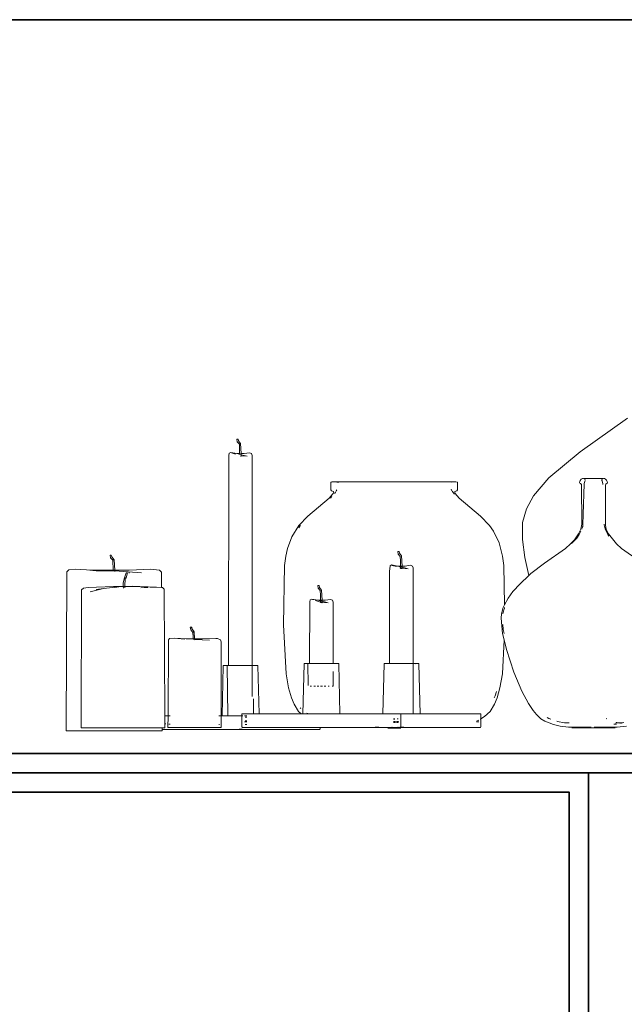
# Model space of a CAD drawing. Units: millimetres. Extents: x 446512 to 447461, y 70395 to 70610.
# Tile 7 of 39: x 446714 to 446730, y 70447 to 70473. Entities that reach past the tile are written whole.
import ezdxf

# ---------------------------------------------------------------- set-up
doc = ezdxf.new("R2010")
doc.units = ezdxf.units.MM
doc.layers.add('A-FURN', color=7, linetype='Continuous', lineweight=35)
doc.layers.add('A-FURN-DECO', color=8, linetype='Continuous', lineweight=13)

msp = doc.modelspace()

# ---------------------------------------------------------------- linework, layer by layer
at = {"layer": 'A-FURN'}
for p, q in [((446686.5728, 70453.3815), (446746.5728, 70453.3815)), ((446729.0084, 70453.3815), (446729.0084, 70433.3815))]:
    msp.add_line(p, q, dxfattribs=at)
for points in [[(446699.4288, 70473.3815), (446746.5728, 70473.3815), (446746.5728, 70453.3815), (446699.4288, 70453.3815)], [(446699.9288, 70472.8815), (446746.0728, 70472.8815), (446746.0728, 70453.8815), (446699.9288, 70453.8815)], [(446686.5728, 70453.3815), (446729.0084, 70453.3815), (446729.0084, 70433.3815), (446686.5728, 70433.3815)], [(446687.0728, 70452.8815), (446728.5084, 70452.8815), (446728.5084, 70433.8815), (446687.0728, 70433.8815)]]:
    msp.add_lwpolyline(points, close=True, dxfattribs=at)
at = {"layer": 'A-FURN-DECO'}
for p, q in [((446728.7945, 70461.6966), (446730.0171, 70462.5633)), ((446719.9441, 70462.0239), (446719.9104, 70462.0221)), ((446719.9188, 70461.9558), (446719.9104, 70462.0221)), ((446719.9756, 70461.8931), (446719.9188, 70461.9558)), ((446719.9519, 70461.9783), (446719.9441, 70462.0239)), ((446720.0049, 70461.9074), (446719.9519, 70461.9783)), ((446719.978, 70461.7795), (446719.9756, 70461.8931)), ((446719.9814, 70461.6492), (446719.978, 70461.7795)), ((446720.0049, 70461.9074), (446720.0223, 70461.6492)), ((446728.7945, 70461.6966), (446727.9781, 70461.0217)), ((446719.6988, 70456.1631), (446719.7022, 70461.6032)), ((446719.7022, 70461.6032), (446719.715, 70461.6578)), ((446719.7565, 70461.6773), (446719.715, 70461.6578)), ((446719.9071, 70461.6494), (446719.7565, 70461.6773)), ((446719.877, 70461.6334), (446719.7704, 70461.6668)), ((446719.7704, 70461.6668), (446719.9071, 70461.6494)), ((446719.9071, 70461.6494), (446719.9814, 70461.6492)), ((446719.982, 70461.63), (446719.9071, 70461.6494)), ((446719.982, 70461.63), (446719.9814, 70461.6492)), ((446720.0243, 70461.619), (446719.982, 70461.63)), ((446719.9821, 70461.6228), (446719.982, 70461.63)), ((446720.01, 70461.5841), (446720.0037, 70461.5844)), ((446720.008, 70461.6492), (446720.0199, 70461.6492)), ((446720.0098, 70461.5932), (446720.0261, 70461.5919)), ((446720.01, 70461.5841), (446720.0267, 70461.5837)), ((446720.0223, 70461.6492), (446720.1003, 70461.6491)), ((446720.0223, 70461.6492), (446720.0243, 70461.619)), ((446720.1784, 70461.5791), (446720.0243, 70461.619)), ((446720.0243, 70461.619), (446720.0256, 70461.5995)), ((446720.0261, 70461.5919), (446720.0267, 70461.5837)), ((446720.0261, 70461.5919), (446720.1784, 70461.5791)), ((446720.1003, 70461.6491), (446720.2369, 70461.6697)), ((446720.2369, 70461.6697), (446720.2923, 70461.6485)), ((446720.2923, 70461.6485), (446720.3052, 70461.5993)), ((446720.3089, 70456.1632), (446720.3052, 70461.5993)), ((446727.5827, 70460.5532), (446727.9781, 70461.0217)), ((446728.7887, 70460.9536), (446728.7747, 70460.9046)), ((446728.8207, 70460.9887), (446728.7887, 70460.9536)), ((446728.8499, 70461.0013), (446728.8207, 70460.9887)), ((446728.8772, 70461.0013), (446728.8499, 70461.0013)), ((446728.8976, 70460.9992), (446728.8772, 70461.0013)), ((446728.8961, 70460.8775), (446728.9208, 70460.9522)), ((446728.8976, 70460.9992), (446728.8991, 70461.0013)), ((446728.8976, 70460.9992), (446728.9159, 70460.9903)), ((446728.8991, 70461.0013), (446729.3721, 70461.0013)), ((446728.9202, 70460.9702), (446728.9159, 70460.9903)), ((446729.3502, 70460.9737), (446729.3477, 70460.9471)), ((446729.3492, 70460.9776), (446729.3509, 70460.9807)), ((446729.3502, 70460.9737), (446729.3492, 70460.9776)), ((446729.3578, 70460.9443), (446729.3502, 70460.9737)), ((446729.3525, 70460.9903), (446729.3508, 70460.9838)), ((446729.3524, 70460.9836), (446729.3569, 70460.992)), ((446729.3736, 70460.9992), (446729.3569, 70460.992)), ((446729.3749, 70460.8785), (446729.3592, 70460.9391)), ((446729.3721, 70461.0013), (446729.3736, 70460.9992)), ((446729.394, 70461.0013), (446729.3736, 70460.9992)), ((446729.4213, 70461.0013), (446729.394, 70461.0013)), ((446729.4459, 70460.9887), (446729.4213, 70461.0013)), ((446729.4459, 70460.9887), (446729.4757, 70460.9645)), ((446729.4925, 70460.9301), (446729.4757, 70460.9645)), ((446729.4925, 70460.9301), (446729.4961, 70460.8996)), ((446722.3491, 70460.9132), (446722.3421, 70460.8983)), ((446722.3453, 70460.7068), (446722.3421, 70460.8983)), ((446722.3453, 70460.7068), (446722.3571, 70460.686)), ((446722.3662, 70460.921), (446722.3491, 70460.9132)), ((446722.3571, 70460.686), (446722.4097, 70460.6657)), ((446722.4195, 70460.921), (446722.3662, 70460.921)), ((446722.3662, 70460.921), (446722.5008, 70460.9114)), ((446722.4311, 70460.922), (446722.4195, 70460.921)), ((446722.4311, 70460.922), (446722.6043, 70460.922)), ((446722.483, 70460.6864), (446722.4986, 70460.7139)), ((446722.5008, 70460.9114), (446722.5021, 70460.9106)), ((446722.5021, 70460.9106), (446722.5091, 70460.9063)), ((446722.5021, 70460.9106), (446722.5457, 70460.9072)), ((446722.5457, 70460.9072), (446722.5479, 70460.9073)), ((446722.8346, 70460.921), (446722.6043, 70460.922)), ((446722.8346, 70460.921), (446723.1792, 70460.921)), ((446723.1792, 70460.921), (446723.5625, 70460.922)), ((446723.5625, 70460.922), (446723.5688, 70460.922)), ((446723.5688, 70460.922), (446723.5748, 70460.922)), ((446723.5748, 70460.922), (446723.9747, 70460.921)), ((446724.4053, 70460.921), (446723.9747, 70460.921)), ((446724.7723, 70460.922), (446724.4053, 70460.921)), ((446724.7898, 70460.922), (446724.7723, 70460.922)), ((446724.7898, 70460.922), (446725.1125, 70460.922)), ((446725.3764, 70460.921), (446725.1125, 70460.922)), ((446725.3764, 70460.921), (446725.5426, 70460.921)), ((446725.452, 70460.9065), (446725.5746, 70460.922)), ((446725.4646, 70460.6981), (446725.4523, 70460.7241)), ((446725.4748, 70460.685), (446725.4646, 70460.6981)), ((446725.5446, 70460.5959), (446725.4822, 70460.6756)), ((446725.5426, 70460.921), (446725.5746, 70460.922)), ((446725.6029, 70460.684), (446725.5502, 70460.6636)), ((446725.5746, 70460.922), (446725.6171, 70460.9078)), ((446725.6169, 70460.7068), (446725.6029, 70460.684)), ((446725.6171, 70460.9078), (446725.6169, 70460.7068)), ((446728.7747, 70460.9046), (446728.7818, 70460.8831)), ((446728.7984, 70460.8735), (446728.7818, 70460.8831)), ((446728.7846, 70460.8865), (446728.7984, 70460.8735)), ((446728.7984, 70460.8735), (446728.8165, 70460.8563)), ((446728.8165, 70460.8563), (446728.8236, 70460.8453)), ((446728.8165, 70460.8563), (446728.8281, 70460.8453)), ((446728.8236, 70460.8453), (446728.8306, 70459.8199)), ((446728.8683, 70460.0694), (446728.8949, 70460.8628)), ((446728.8683, 70460.0694), (446728.898, 70460.862)), ((446729.3752, 70460.8691), (446729.3749, 70460.8785)), ((446729.3761, 70460.8439), (446729.3759, 70460.8497)), ((446729.4475, 70460.8431), (446729.444, 70459.7861)), ((446729.4475, 70460.8431), (446729.4529, 70460.8582)), ((446729.4529, 70460.8582), (446729.4894, 70460.8831)), ((446729.4894, 70460.8831), (446729.4961, 70460.8996)), ((446722.2982, 70460.4984), (446721.7473, 70460.0316)), ((446722.396, 70460.6047), (446722.2982, 70460.4984)), ((446722.3339, 70460.4984), (446722.3632, 70460.5266)), ((446722.3708, 70460.5354), (446722.3632, 70460.5266)), ((446722.416, 70460.6431), (446722.396, 70460.6047)), ((446722.4097, 70460.6657), (446722.416, 70460.6431)), ((446722.4502, 70460.6286), (446722.4382, 70460.6146)), ((446722.4502, 70460.6286), (446722.473, 70460.6689)), ((446725.5502, 70460.6636), (446725.5453, 70460.6516)), ((446725.5453, 70460.6516), (446725.5562, 70460.6199)), ((446725.5562, 70460.6199), (446725.664, 70460.4984)), ((446725.664, 70460.4984), (446726.2149, 70460.0316)), ((446727.4014, 70460.2208), (446727.5827, 70460.5532)), ((446727.4014, 70460.2208), (446727.3011, 70459.8693)), ((446721.7473, 70460.0316), (446721.5179, 70459.7851)), ((446726.2149, 70460.0316), (446726.4443, 70459.7851)), ((446728.8683, 70460.0694), (446728.8587, 70459.813)), ((446721.5179, 70459.7851), (446721.3347, 70459.4924)), ((446721.5131, 70459.7239), (446721.5432, 70459.7682)), ((446721.5432, 70459.7682), (446721.5573, 70459.7851)), ((446726.4443, 70459.7851), (446726.5455, 70459.6402)), ((446727.3011, 70459.8693), (446727.2951, 70459.4275)), ((446728.7483, 70459.5707), (446728.8051, 70459.6966)), ((446728.8306, 70459.8199), (446728.8051, 70459.6966)), ((446728.8368, 70459.6996), (446728.8326, 70459.6907)), ((446728.8575, 70459.7807), (446728.8409, 70459.715)), ((446728.8564, 70459.752), (446728.8575, 70459.7807)), ((446728.8588, 70459.786), (446728.8575, 70459.7807)), ((446728.8587, 70459.813), (446728.8588, 70459.786)), ((446729.4108, 70459.801), (446729.4101, 70459.8199)), ((446729.4338, 70459.7009), (446729.4108, 70459.801)), ((446729.5022, 70459.5548), (446729.4338, 70459.7009)), ((446729.444, 70459.7861), (446729.4661, 70459.6966)), ((446729.4661, 70459.6966), (446729.5229, 70459.5707)), ((446721.3347, 70459.4924), (446721.2205, 70459.1885)), ((446726.5455, 70459.6402), (446726.6922, 70459.3418)), ((446727.3592, 70458.9579), (446727.2951, 70459.4275)), ((446728.6407, 70459.4164), (446728.5404, 70459.3091)), ((446728.5656, 70459.3206), (446728.7087, 70459.464)), ((446728.6407, 70459.4164), (446728.7483, 70459.5707)), ((446728.769, 70459.5548), (446728.7087, 70459.464)), ((446728.8078, 70459.6377), (446728.769, 70459.5548)), ((446729.5334, 70459.513), (446729.5022, 70459.5548)), ((446729.5229, 70459.5707), (446729.7308, 70459.3091)), ((446721.2205, 70459.1885), (446721.1771, 70458.9933)), ((446726.6922, 70459.3418), (446726.7851, 70458.9933)), ((446728.4101, 70459.1958), (446727.8647, 70458.8154)), ((446728.5404, 70459.3091), (446728.4101, 70459.1958)), ((446729.8611, 70459.1958), (446729.7308, 70459.3091)), ((446730.4065, 70458.8154), (446729.8611, 70459.1958)), ((446716.6354, 70459.0201), (446716.6571, 70459.0212)), ((446716.6354, 70459.0201), (446716.6442, 70458.9513)), ((446716.6442, 70458.9513), (446716.7034, 70458.8861)), ((446716.6787, 70458.9748), (446716.6571, 70459.0212)), ((446716.6866, 70458.9642), (446716.6787, 70458.9748)), ((446716.7339, 70458.901), (446716.6866, 70458.9642)), ((446716.7224, 70458.8952), (446716.6866, 70458.9642)), ((446716.7034, 70458.8861), (446716.7224, 70458.8952)), ((446716.7224, 70458.8952), (446716.7339, 70458.901)), ((446716.752, 70458.632), (446716.7339, 70458.901)), ((446721.1771, 70458.9933), (446721.1469, 70458.754)), ((446724.1064, 70459.1159), (446724.0725, 70459.1141)), ((446724.0809, 70459.0472), (446724.0725, 70459.1141)), ((446724.1382, 70458.984), (446724.0809, 70459.0472)), ((446724.1143, 70459.0699), (446724.1064, 70459.1159)), ((446724.1678, 70458.9984), (446724.1143, 70459.0699)), ((446724.1406, 70458.8694), (446724.1382, 70458.984)), ((446724.1678, 70458.9984), (446724.1853, 70458.7377)), ((446726.7851, 70458.9933), (446726.8153, 70458.754)), ((446727.4673, 70458.4954), (446727.3592, 70458.9579)), ((446715.5105, 70458.5841), (446715.5626, 70458.641)), ((446715.5626, 70458.641), (446715.7315, 70458.6612)), ((446715.7315, 70458.6612), (446716.0257, 70458.6369)), ((446716.0257, 70458.6369), (446716.3433, 70458.6322)), ((446716.0257, 70458.6369), (446716.2746, 70458.615)), ((446716.3433, 70458.6322), (446716.7096, 70458.632)), ((446716.7034, 70458.8861), (446716.7096, 70458.632)), ((446716.7096, 70458.632), (446716.71, 70458.6145)), ((446716.7187, 70458.632), (446716.752, 70458.632)), ((446716.752, 70458.632), (446717.1286, 70458.6319)), ((446716.7533, 70458.6131), (446716.752, 70458.632)), ((446717.6839, 70458.6534), (446717.1286, 70458.6319)), ((446717.6839, 70458.6534), (446717.9093, 70458.6313)), ((446721.1469, 70458.754), (446721.119, 70457.2186)), ((446723.8582, 70458.5941), (446723.8754, 70458.7468)), ((446723.9173, 70458.7664), (446723.8754, 70458.7468)), ((446723.9173, 70458.7664), (446724.0691, 70458.7374)), ((446723.9313, 70458.7559), (446724.0691, 70458.7374)), ((446724.0388, 70458.7222), (446723.9313, 70458.7559)), ((446724.1441, 70458.7376), (446724.0691, 70458.7374)), ((446724.1446, 70458.7181), (446724.0691, 70458.7374)), ((446724.1454, 70458.6888), (446724.1244, 70458.6954)), ((446724.1441, 70458.7376), (446724.1406, 70458.8694)), ((446724.1853, 70458.7377), (446724.1441, 70458.7376)), ((446724.1446, 70458.7181), (446724.1441, 70458.7376)), ((446724.1448, 70458.7115), (446724.1446, 70458.7181)), ((446724.1873, 70458.7072), (446724.1446, 70458.7181)), ((446724.1454, 70458.6888), (446724.145, 70458.7021)), ((446724.1665, 70458.6822), (446724.1454, 70458.6888)), ((446724.1458, 70458.6738), (446724.1454, 70458.6888)), ((446724.1729, 70458.6724), (446724.1458, 70458.6738)), ((446724.1891, 70458.6803), (446724.1665, 70458.6822)), ((446724.1729, 70458.6724), (446724.1897, 70458.672)), ((446724.2639, 70458.7379), (446724.1853, 70458.7377)), ((446724.1853, 70458.7377), (446724.1873, 70458.7072)), ((446724.1873, 70458.7072), (446724.1886, 70458.6881)), ((446724.3427, 70458.6674), (446724.1873, 70458.7072)), ((446724.1891, 70458.6803), (446724.1897, 70458.672)), ((446724.3427, 70458.6674), (446724.1891, 70458.6803)), ((446724.4017, 70458.7588), (446724.2639, 70458.7379)), ((446724.4576, 70458.7374), (446724.4017, 70458.7588)), ((446724.4705, 70458.6877), (446724.4576, 70458.7374)), ((446724.4724, 70456.2151), (446724.4705, 70458.6877)), ((446726.8153, 70458.754), (446726.8338, 70457.7327)), ((446727.5189, 70458.543), (446727.8647, 70458.8154)), ((446715.4932, 70454.4707), (446715.5105, 70458.5841)), ((446716.2746, 70458.615), (446716.2883, 70458.6148)), ((446716.2883, 70458.6148), (446716.71, 70458.6145)), ((446716.71, 70458.6145), (446716.7359, 70458.6145)), ((446716.7359, 70458.6145), (446716.7533, 70458.6131)), ((446716.7533, 70458.6131), (446717.4462, 70458.559)), ((446716.7541, 70458.6003), (446716.7533, 70458.6131)), ((446716.9685, 70458.3005), (446717.004, 70458.4341)), ((446717.004, 70458.4341), (446717.0495, 70458.5607)), ((446717.0229, 70458.425), (446717.0178, 70458.2115)), ((446717.0245, 70458.4398), (446717.0229, 70458.425)), ((446717.0229, 70458.425), (446717.042, 70458.425)), ((446717.042, 70458.425), (446717.0475, 70458.434)), ((446717.0475, 70458.434), (446717.0856, 70458.56)), ((446717.0495, 70458.5607), (446717.0856, 70458.56)), ((446717.1161, 70458.5661), (446717.1347, 70458.5657)), ((446717.9614, 70458.58), (446717.9093, 70458.6313)), ((446717.963, 70458.1808), (446717.9614, 70458.58)), ((446723.8582, 70456.2151), (446723.8582, 70458.5941)), ((446727.2355, 70458.2815), (446727.4673, 70458.4954)), ((446727.4673, 70458.4954), (446727.5189, 70458.543)), ((446715.8817, 70454.5456), (446715.8968, 70458.1227)), ((446715.9421, 70458.1689), (446715.8968, 70458.1227)), ((446716.0693, 70458.1802), (446715.9421, 70458.1689)), ((446716.7205, 70458.2113), (446716.0693, 70458.1802)), ((446716.1194, 70458.0708), (446716.4619, 70458.1529)), ((446716.2717, 70458.1312), (446716.4619, 70458.1529)), ((446716.8597, 70458.2036), (446716.4619, 70458.1529)), ((446716.7205, 70458.2113), (446716.9736, 70458.2114)), ((446716.759, 70458.1855), (446716.8597, 70458.2036)), ((446716.8597, 70458.2036), (446716.9738, 70458.207)), ((446716.9736, 70458.2114), (446716.9685, 70458.3005)), ((446716.9736, 70458.2114), (446716.9777, 70458.2114)), ((446716.9738, 70458.207), (446716.9736, 70458.2114)), ((446716.9738, 70458.207), (446717.0177, 70458.2083)), ((446716.9761, 70458.1671), (446716.9738, 70458.207)), ((446717.0004, 70458.2115), (446717.0178, 70458.2115)), ((446717.0177, 70458.2083), (446717.0167, 70458.1721)), ((446717.0177, 70458.2083), (446717.1242, 70458.2115)), ((446717.0178, 70458.2115), (446717.0177, 70458.2083)), ((446717.0178, 70458.2115), (446717.1242, 70458.2115)), ((446717.1242, 70458.2115), (446717.2075, 70458.214)), ((446717.1242, 70458.2115), (446717.2775, 70458.2116)), ((446717.2075, 70458.214), (446717.2775, 70458.2116)), ((446717.2775, 70458.2116), (446717.7488, 70458.1951)), ((446717.2775, 70458.2116), (446717.4044, 70458.2116)), ((446717.4044, 70458.2116), (446717.8303, 70458.1954)), ((446717.4299, 70458.1719), (446717.6043, 70458.1821)), ((446717.6751, 70458.1863), (446717.8303, 70458.1954)), ((446717.8303, 70458.1954), (446717.7488, 70458.1951)), ((446717.8303, 70458.1954), (446717.963, 70458.1808)), ((446717.963, 70458.1808), (446717.9858, 70458.1808)), ((446717.9858, 70458.1808), (446718.0312, 70458.1354)), ((446718.0312, 70458.1354), (446718.045, 70454.8578)), ((446722.0386, 70458.2326), (446722.0047, 70458.2307)), ((446722.0131, 70458.164), (446722.0047, 70458.2307)), ((446722.0702, 70458.1009), (446722.0131, 70458.164)), ((446722.0464, 70458.1866), (446722.0386, 70458.2326)), ((446722.0998, 70458.1153), (446722.0464, 70458.1866)), ((446727.0519, 70458.0782), (446727.2355, 70458.2815)), ((446721.808, 70457.8642), (446721.8498, 70457.8837)), ((446721.8498, 70457.8837), (446722.0013, 70457.8556)), ((446721.8638, 70457.8732), (446722.0013, 70457.8556)), ((446722.0726, 70457.9866), (446722.0702, 70458.1009)), ((446722.0761, 70457.8555), (446722.0726, 70457.9866)), ((446722.0998, 70458.1153), (446722.1172, 70457.8555)), ((446722.1957, 70457.8554), (446722.3332, 70457.8761)), ((446722.389, 70457.8548), (446722.3332, 70457.8761)), ((446726.9252, 70457.9066), (446726.8338, 70457.7327)), ((446727.0519, 70458.0782), (446726.9252, 70457.9066)), ((446721.792, 70456.2151), (446721.7951, 70457.8092)), ((446721.7951, 70457.8092), (446721.808, 70457.8642)), ((446721.9427, 70457.8485), (446722.0774, 70457.8063)), ((446722.0013, 70457.8556), (446722.0761, 70457.8555)), ((446722.0013, 70457.8556), (446722.0766, 70457.8361)), ((446722.0761, 70457.8555), (446722.1172, 70457.8555)), ((446722.0766, 70457.8361), (446722.0761, 70457.8555)), ((446722.0766, 70457.8361), (446722.1192, 70457.8251)), ((446722.0774, 70457.8063), (446722.0766, 70457.8361)), ((446722.0774, 70457.8063), (446722.0985, 70457.7997)), ((446722.0778, 70457.7914), (446722.0774, 70457.8063)), ((446722.1049, 70457.79), (446722.0778, 70457.7914)), ((446722.1211, 70457.7978), (446722.0985, 70457.7997)), ((446722.1049, 70457.79), (446722.1216, 70457.7896)), ((446722.1172, 70457.8555), (446722.1957, 70457.8554)), ((446722.1172, 70457.8555), (446722.1192, 70457.8251)), ((446722.1192, 70457.8251), (446722.2743, 70457.7849)), ((446722.1192, 70457.8251), (446722.1211, 70457.7978)), ((446722.2743, 70457.7849), (446722.1211, 70457.7978)), ((446722.1211, 70457.7978), (446722.1216, 70457.7896)), ((446722.4019, 70457.8053), (446722.389, 70457.8548)), ((446722.4019, 70457.8053), (446722.405, 70456.2151)), ((446726.7531, 70457.4982), (446726.7992, 70457.6668)), ((446726.8338, 70457.7327), (446726.7992, 70457.6668)), ((446726.8355, 70457.6426), (446726.8171, 70457.6055)), ((446726.835, 70457.6668), (446726.837, 70457.6484)), ((446726.837, 70457.6484), (446726.8354, 70457.6449)), ((446726.8354, 70457.6449), (446726.8355, 70457.6426)), ((446726.7448, 70457.3867), (446726.7531, 70457.4982)), ((446726.7448, 70457.3867), (446726.7852, 70456.9946)), ((446726.7902, 70457.4982), (446726.8171, 70457.6055)), ((446718.7295, 70457.1576), (446718.7075, 70457.1558)), ((446718.7164, 70457.0871), (446718.7075, 70457.1558)), ((446718.7295, 70457.1576), (446718.7428, 70457.1581)), ((446718.7495, 70457.1187), (446718.7295, 70457.1576)), ((446718.7495, 70457.1187), (446718.7428, 70457.1581)), ((446718.7509, 70457.1106), (446718.7495, 70457.1187)), ((446718.7598, 70457.0987), (446718.7495, 70457.1187)), ((446718.7598, 70457.0987), (446718.7509, 70457.1106)), ((446721.119, 70457.2186), (446721.1834, 70455.9479)), ((446726.7872, 70457.222), (446726.8035, 70457.0922)), ((446718.1394, 70456.8302), (446718.1682, 70456.8616)), ((446718.2925, 70456.8668), (446718.1682, 70456.8616)), ((446718.5676, 70456.8447), (446718.2925, 70456.8668)), ((446718.5988, 70456.8568), (446718.2925, 70456.8668)), ((446718.2925, 70456.8668), (446718.7797, 70456.8412)), ((446718.7793, 70456.8567), (446718.5988, 70456.8568)), ((446718.7164, 70457.0871), (446718.7756, 70457.0219)), ((446718.7946, 70457.031), (446718.7598, 70457.0987)), ((446718.8061, 70457.0368), (446718.7598, 70457.0987)), ((446718.7946, 70457.031), (446718.7756, 70457.0219)), ((446718.7784, 70456.9061), (446718.7756, 70457.0219)), ((446718.778, 70456.9035), (446718.7784, 70456.9061)), ((446718.778, 70456.9035), (446718.7793, 70456.8567)), ((446718.7793, 70456.8567), (446718.7797, 70456.8412)), ((446718.8182, 70456.8567), (446718.7793, 70456.8567)), ((446718.8061, 70457.0368), (446718.7946, 70457.031)), ((446718.8182, 70456.8567), (446718.8061, 70457.0368)), ((446718.8193, 70456.8398), (446718.8182, 70456.8567)), ((446719.0321, 70456.8566), (446718.8182, 70456.8567)), ((446719.3696, 70456.8619), (446719.0321, 70456.8566)), ((446719.4116, 70456.8598), (446719.3696, 70456.8619)), ((446719.4915, 70456.828), (446719.4116, 70456.8598)), ((446726.8235, 70456.8308), (446726.7852, 70456.9946)), ((446726.8035, 70457.0922), (446726.8258, 70456.9946)), ((446718.1311, 70454.8578), (446718.1394, 70456.8302)), ((446718.7797, 70456.8412), (446718.8155, 70456.8401)), ((446718.8193, 70456.8398), (446718.8155, 70456.8401)), ((446719.2073, 70456.8164), (446718.8193, 70456.8398)), ((446718.8214, 70456.8095), (446718.8213, 70456.8112)), ((446719.5011, 70456.7748), (446719.4915, 70456.828)), ((446719.5011, 70456.7748), (446719.5011, 70454.8578)), ((446726.8235, 70456.8308), (446726.7788, 70455.9479)), ((446726.8836, 70456.5742), (446726.8235, 70456.8308)), ((446727.0748, 70455.9925), (446726.8836, 70456.5742)), ((446719.5279, 70454.8578), (446719.5578, 70456.1587)), ((446719.5578, 70456.1587), (446719.563, 70456.1631)), ((446719.5894, 70456.1631), (446719.563, 70456.1631)), ((446719.5973, 70456.1632), (446719.5894, 70456.1631)), ((446719.6042, 70456.1631), (446719.5973, 70456.1632)), ((446719.6064, 70456.1631), (446719.6042, 70456.1631)), ((446719.6089, 70456.1632), (446719.6064, 70456.1631)), ((446719.6245, 70456.1631), (446719.6089, 70456.1632)), ((446719.6245, 70456.1631), (446719.6397, 70456.1632)), ((446719.6397, 70456.1632), (446719.6479, 70456.1632)), ((446719.6479, 70456.1632), (446719.6517, 70456.1631)), ((446719.6517, 70456.1631), (446719.6576, 70456.1632)), ((446719.6576, 70456.1632), (446719.6768, 70454.8578)), ((446719.6576, 70456.1632), (446719.6674, 70456.1632)), ((446719.6761, 70456.1631), (446719.6674, 70456.1632)), ((446719.6783, 70456.1632), (446719.6761, 70456.1631)), ((446719.6988, 70456.1631), (446719.6783, 70456.1632)), ((446719.6988, 70456.1631), (446719.708, 70456.1632)), ((446719.6988, 70456.1587), (446719.6988, 70456.1631)), ((446719.708, 70456.1632), (446719.7106, 70456.1631)), ((446719.7106, 70456.1631), (446719.7228, 70456.1631)), ((446719.7228, 70456.1631), (446719.7272, 70456.1632)), ((446719.7272, 70456.1632), (446719.7304, 70456.1632)), ((446719.7304, 70456.1632), (446719.7469, 70456.1632)), ((446719.7574, 70456.1632), (446719.7469, 70456.1632)), ((446719.7574, 70456.1632), (446719.7735, 70456.1632)), ((446719.7766, 70456.1631), (446719.7735, 70456.1632)), ((446719.7794, 70456.1632), (446719.7766, 70456.1631)), ((446719.781, 70456.1631), (446719.7794, 70456.1632)), ((446719.7832, 70456.1632), (446719.781, 70456.1631)), ((446719.7881, 70456.1631), (446719.7832, 70456.1632)), ((446719.7881, 70456.1631), (446719.8002, 70456.1632)), ((446719.8196, 70456.1631), (446719.8002, 70456.1632)), ((446719.8196, 70456.1631), (446719.8593, 70456.1632)), ((446719.9019, 70456.1631), (446719.8593, 70456.1632)), ((446719.9019, 70456.1631), (446719.9241, 70456.1632)), ((446719.9241, 70456.1632), (446719.9883, 70456.1631)), ((446719.9883, 70456.1631), (446719.992, 70456.1632)), ((446719.992, 70456.1632), (446720.0264, 70456.1632)), ((446720.032, 70456.1631), (446720.0264, 70456.1632)), ((446720.032, 70456.1631), (446720.0943, 70456.1632)), ((446720.1182, 70456.1631), (446720.0943, 70456.1632)), ((446720.1182, 70456.1631), (446720.1588, 70456.1632)), ((446720.2002, 70456.1631), (446720.1588, 70456.1632)), ((446720.2002, 70456.1631), (446720.2176, 70456.1632)), ((446720.2176, 70456.1632), (446720.2386, 70456.1631)), ((446720.2386, 70456.1631), (446720.2682, 70456.1632)), ((446720.2682, 70456.1632), (446720.2754, 70456.1632)), ((446720.2941, 70456.1632), (446720.2754, 70456.1632)), ((446720.2941, 70456.1632), (446720.3038, 70456.1631)), ((446720.3038, 70456.1631), (446720.3089, 70456.1632)), ((446720.3091, 70455.3578), (446720.3089, 70456.1632)), ((446720.3115, 70456.1632), (446720.3089, 70456.1632)), ((446720.3207, 70456.1632), (446720.3115, 70456.1632)), ((446720.3222, 70456.1632), (446720.3207, 70456.1632)), ((446720.3235, 70456.1632), (446720.3222, 70456.1632)), ((446720.3235, 70456.1632), (446720.3249, 70456.1632)), ((446720.3296, 70456.1632), (446720.3249, 70456.1632)), ((446720.331, 70456.1632), (446720.3296, 70456.1632)), ((446720.3333, 70456.1632), (446720.331, 70456.1632)), ((446720.3356, 70456.1631), (446720.3333, 70456.1632)), ((446720.339, 70456.1631), (446720.3356, 70456.1631)), ((446720.3427, 70456.1632), (446720.339, 70456.1631)), ((446720.3444, 70456.1632), (446720.3427, 70456.1632)), ((446720.3444, 70456.1632), (446720.3478, 70456.1632)), ((446720.3456, 70456.1632), (446720.3444, 70456.1632)), ((446720.3478, 70456.1632), (446720.3456, 70456.1632)), ((446720.3478, 70456.1632), (446720.3503, 70456.1632)), ((446720.3538, 70456.1632), (446720.3503, 70456.1632)), ((446720.3575, 70456.1632), (446720.3538, 70456.1632)), ((446720.3575, 70456.1632), (446720.3575, 70456.1587)), ((446720.361, 70456.1632), (446720.3575, 70456.1632)), ((446720.3635, 70456.1631), (446720.361, 70456.1632)), ((446720.3809, 70456.1632), (446720.3635, 70456.1631)), ((446720.3872, 70456.1632), (446720.3809, 70456.1632)), ((446720.3906, 70456.1631), (446720.3872, 70456.1632)), ((446720.3926, 70456.1632), (446720.3906, 70456.1631)), ((446720.3926, 70456.1632), (446720.452, 70456.1631)), ((446720.4574, 70456.1587), (446720.452, 70456.1631)), ((446720.4861, 70454.9097), (446720.4574, 70456.1587)), ((446721.6183, 70454.9097), (446721.6482, 70456.2106)), ((446721.6482, 70456.2106), (446721.6536, 70456.2151)), ((446721.6536, 70456.2151), (446721.7072, 70456.2151)), ((446721.7072, 70456.2151), (446721.7119, 70456.2151)), ((446721.7119, 70456.2151), (446721.7149, 70456.2151)), ((446721.7149, 70456.2151), (446721.7175, 70456.2151)), ((446721.7175, 70456.2151), (446721.7188, 70456.2151)), ((446721.7188, 70456.2151), (446721.726, 70456.2151)), ((446721.726, 70456.2151), (446721.739, 70456.2151)), ((446721.739, 70456.2151), (446721.741, 70456.2152)), ((446721.741, 70456.2152), (446721.7438, 70456.2151)), ((446721.7438, 70456.2151), (446721.7481, 70456.2152)), ((446721.7481, 70456.2152), (446721.7565, 70455.6418)), ((446721.7481, 70456.2152), (446721.7585, 70456.2152)), ((446721.7585, 70456.2152), (446721.7699, 70456.2151)), ((446721.7699, 70456.2151), (446721.7806, 70456.2152)), ((446721.7806, 70456.2152), (446721.782, 70456.2152)), ((446721.7901, 70456.2151), (446721.782, 70456.2152)), ((446721.792, 70456.2151), (446721.7901, 70456.2151)), ((446721.792, 70456.2106), (446721.792, 70456.2151)), ((446721.792, 70456.2151), (446721.8162, 70456.2151)), ((446721.8162, 70456.2151), (446721.8176, 70456.2152)), ((446721.8176, 70456.2152), (446721.8639, 70456.2152)), ((446721.8713, 70456.2151), (446721.8639, 70456.2152)), ((446721.8713, 70456.2151), (446721.8906, 70456.2152)), ((446721.9923, 70456.2151), (446721.8906, 70456.2152)), ((446721.9923, 70456.2151), (446722.0144, 70456.2152)), ((446722.0787, 70456.2151), (446722.0144, 70456.2152)), ((446722.0787, 70456.2151), (446722.0824, 70456.2152)), ((446722.0824, 70456.2152), (446722.1168, 70456.2152)), ((446722.1223, 70456.2151), (446722.1168, 70456.2152)), ((446722.1223, 70456.2151), (446722.1847, 70456.2152)), ((446722.2086, 70456.2151), (446722.1847, 70456.2152)), ((446722.3079, 70456.2152), (446722.2086, 70456.2151)), ((446722.3079, 70456.2152), (446722.3289, 70456.2151)), ((446722.3289, 70456.2151), (446722.3344, 70456.2152)), ((446722.3344, 70456.2152), (446722.3807, 70456.2151)), ((446722.3807, 70456.2151), (446722.405, 70456.2151)), ((446722.405, 70456.2151), (446722.405, 70456.2106)), ((446722.4294, 70456.2151), (446722.405, 70456.2151)), ((446722.4294, 70456.2151), (446722.4321, 70456.2151)), ((446722.4321, 70456.2151), (446722.4341, 70456.2151)), ((446722.4341, 70456.2151), (446722.4442, 70456.2152)), ((446722.4479, 70456.2152), (446722.4442, 70456.2152)), ((446722.4479, 70456.2152), (446722.4478, 70456.2106)), ((446722.4783, 70456.2151), (446722.4479, 70456.2152)), ((446722.4783, 70456.2151), (446722.481, 70456.2151)), ((446722.487, 70456.2151), (446722.481, 70456.2151)), ((446722.4992, 70456.2151), (446722.487, 70456.2151)), ((446722.4992, 70456.2151), (446722.5426, 70456.2151)), ((446722.5477, 70456.2106), (446722.5426, 70456.2151)), ((446722.5776, 70454.9097), (446722.5477, 70456.2106)), ((446723.6892, 70454.9097), (446723.7191, 70456.2106)), ((446723.7191, 70456.2106), (446723.7245, 70456.2151)), ((446723.7245, 70456.2151), (446723.7786, 70456.2151)), ((446723.7834, 70456.2151), (446723.7786, 70456.2151)), ((446723.8032, 70456.2151), (446723.7834, 70456.2151)), ((446723.8099, 70456.2151), (446723.8032, 70456.2151)), ((446723.813, 70456.2151), (446723.8099, 70456.2151)), ((446723.8191, 70456.2152), (446723.813, 70456.2151)), ((446723.8191, 70456.2152), (446723.819, 70456.2106)), ((446723.8191, 70456.2152), (446723.8295, 70456.2152)), ((446723.8374, 70456.2151), (446723.8295, 70456.2152)), ((446723.8435, 70456.2152), (446723.8374, 70456.2151)), ((446723.8515, 70456.2152), (446723.8435, 70456.2152)), ((446723.8529, 70456.2152), (446723.8515, 70456.2152)), ((446723.8582, 70456.2151), (446723.8529, 70456.2152)), ((446723.8676, 70456.2152), (446723.8582, 70456.2151)), ((446723.8582, 70456.2106), (446723.8582, 70456.2151)), ((446723.8719, 70456.2151), (446723.8676, 70456.2152)), ((446723.8719, 70456.2151), (446723.878, 70456.2151)), ((446723.878, 70456.2151), (446723.884, 70456.2151)), ((446723.884, 70456.2151), (446723.8885, 70456.2152)), ((446723.8885, 70456.2152), (446723.9058, 70456.2151)), ((446723.9058, 70456.2151), (446723.9104, 70456.2152)), ((446723.9104, 70456.2152), (446723.9485, 70456.2151)), ((446723.9485, 70456.2151), (446723.9589, 70456.2152)), ((446723.9589, 70456.2152), (446723.9615, 70456.2152)), ((446723.9809, 70456.2151), (446723.9615, 70456.2152)), ((446723.9809, 70456.2151), (446723.9902, 70456.2152)), ((446724.0099, 70456.2151), (446723.9902, 70456.2152)), ((446724.0099, 70456.2151), (446724.0524, 70456.2152)), ((446724.0632, 70456.2151), (446724.0524, 70456.2152)), ((446724.0632, 70456.2151), (446724.1191, 70456.2152)), ((446724.1496, 70456.2151), (446724.1191, 70456.2152)), ((446724.1496, 70456.2151), (446724.1877, 70456.2152)), ((446724.2367, 70456.2151), (446724.1877, 70456.2152)), ((446724.2367, 70456.2151), (446724.2556, 70456.2152)), ((446724.2556, 70456.2152), (446724.3201, 70456.2152)), ((446724.3218, 70456.2151), (446724.3201, 70456.2152)), ((446724.3218, 70456.2151), (446724.3476, 70456.2152)), ((446724.3476, 70456.2152), (446724.3698, 70456.2151)), ((446724.3789, 70456.2152), (446724.3698, 70456.2151)), ((446724.3833, 70456.2151), (446724.3789, 70456.2152)), ((446724.3833, 70456.2151), (446724.3999, 70456.2151)), ((446724.3999, 70456.2151), (446724.4295, 70456.2152)), ((446724.464, 70456.2151), (446724.4295, 70456.2152)), ((446724.4659, 70456.2151), (446724.464, 70456.2151)), ((446724.4697, 70456.2151), (446724.4659, 70456.2151)), ((446724.4724, 70456.2151), (446724.4697, 70456.2151)), ((446724.4734, 70454.9097), (446724.4724, 70456.2151)), ((446724.4752, 70456.2151), (446724.4724, 70456.2151)), ((446724.4778, 70456.2151), (446724.4752, 70456.2151)), ((446724.4793, 70456.2151), (446724.4778, 70456.2151)), ((446724.4831, 70456.2151), (446724.4793, 70456.2151)), ((446724.4849, 70456.2152), (446724.4831, 70456.2151)), ((446724.4873, 70456.2151), (446724.4849, 70456.2152)), ((446724.489, 70456.2151), (446724.4873, 70456.2151)), ((446724.4969, 70456.2151), (446724.489, 70456.2151)), ((446724.4993, 70456.2152), (446724.4969, 70456.2151)), ((446724.4993, 70456.2152), (446724.5018, 70456.2151)), ((446724.5018, 70456.2151), (446724.5152, 70456.2152)), ((446724.5189, 70456.2152), (446724.5152, 70456.2152)), ((446724.5189, 70456.2152), (446724.5188, 70456.2106)), ((446724.5279, 70456.2151), (446724.5189, 70456.2152)), ((446724.5303, 70456.2151), (446724.5279, 70456.2151)), ((446724.5342, 70456.2151), (446724.5303, 70456.2151)), ((446724.5365, 70456.2152), (446724.5342, 70456.2151)), ((446724.5493, 70456.2151), (446724.5365, 70456.2152)), ((446724.5613, 70456.2151), (446724.5493, 70456.2151)), ((446724.5668, 70456.2151), (446724.5613, 70456.2151)), ((446724.5668, 70456.2151), (446724.6133, 70456.2151)), ((446724.6187, 70456.2106), (446724.6133, 70456.2151)), ((446724.6486, 70454.9097), (446724.6187, 70456.2106)), ((446721.1834, 70455.9479), (446721.2475, 70455.5851)), ((446722.4054, 70456.007), (446722.4061, 70455.6258)), ((446726.7788, 70455.9479), (446726.7147, 70455.5851)), ((446727.0748, 70455.9925), (446727.2856, 70455.4981)), ((446721.2475, 70455.5851), (446721.3203, 70455.3274)), ((446721.8034, 70455.6258), (446721.8399, 70455.6258)), ((446721.9443, 70455.6258), (446721.9022, 70455.6258)), ((446722.0326, 70455.6258), (446721.9879, 70455.6258)), ((446722.0779, 70455.6258), (446722.1234, 70455.6258)), ((446722.2133, 70455.6258), (446722.1687, 70455.6258)), ((446722.2987, 70455.6258), (446722.2743, 70455.6258)), ((446722.4061, 70455.6258), (446722.3763, 70455.6258)), ((446726.7147, 70455.5851), (446726.6419, 70455.3274)), ((446721.3203, 70455.3274), (446721.3893, 70455.1589)), ((446726.5668, 70455.3274), (446726.592, 70455.3759)), ((446726.6419, 70455.3274), (446726.5729, 70455.1589)), ((446726.592, 70455.3759), (446726.6307, 70455.4902)), ((446727.4568, 70455.1775), (446727.2856, 70455.4981)), ((446720.3449, 70455.3023), (446720.3391, 70454.9097)), ((446721.3893, 70455.1589), (446721.5027, 70454.9746)), ((446721.5697, 70455.0499), (446721.5495, 70455.0689)), ((446726.5729, 70455.1589), (446726.4595, 70454.9746)), ((446727.4568, 70455.1775), (446727.5727, 70455.0013)), ((446718.045, 70454.8578), (446718.0459, 70454.6495)), ((446718.045, 70454.8578), (446718.1311, 70454.8578)), ((446718.1299, 70454.561), (446718.1311, 70454.8578)), ((446718.1311, 70454.8578), (446718.1852, 70454.8578)), ((446719.4457, 70454.8578), (446719.5011, 70454.8578)), ((446719.5011, 70454.8578), (446719.5011, 70454.561)), ((446719.5011, 70454.8578), (446719.5279, 70454.8578)), ((446719.5279, 70454.8578), (446719.6768, 70454.8578)), ((446720.0427, 70454.8578), (446719.6768, 70454.8578)), ((446720.0423, 70454.5773), (446720.0427, 70454.8578)), ((446720.0427, 70454.8578), (446720.0428, 70454.9097)), ((446720.0427, 70454.8578), (446720.0661, 70454.8578)), ((446720.0428, 70454.9097), (446720.0608, 70454.9097)), ((446720.0636, 70454.9096), (446720.0608, 70454.9097)), ((446720.0636, 70454.9096), (446720.0662, 70454.9097)), ((446720.0662, 70454.9097), (446720.0666, 70454.9064)), ((446720.0662, 70454.9097), (446720.1073, 70454.9097)), ((446720.1675, 70454.8578), (446720.1072, 70454.8578)), ((446720.1073, 70454.9097), (446720.1187, 70454.9096)), ((446720.1187, 70454.9096), (446720.1275, 70454.9096)), ((446720.1272, 70454.8261), (446720.1675, 70454.8261)), ((446720.1275, 70454.9096), (446720.1553, 70454.9097)), ((446720.3391, 70454.9097), (446720.1553, 70454.9097)), ((446720.4861, 70454.9097), (446720.3391, 70454.9097)), ((446721.571, 70454.9097), (446720.4861, 70454.9097)), ((446721.5027, 70454.9746), (446721.571, 70454.9097)), ((446721.571, 70454.9097), (446721.6183, 70454.9097)), ((446722.5776, 70454.9097), (446721.6183, 70454.9097)), ((446721.7443, 70454.9174), (446721.7225, 70454.929)), ((446723.6892, 70454.9097), (446722.5776, 70454.9097)), ((446723.9662, 70454.9097), (446723.6892, 70454.9097)), ((446723.9702, 70454.9118), (446723.9662, 70454.9097)), ((446723.9702, 70454.9118), (446723.9663, 70454.9112)), ((446723.9752, 70454.9097), (446723.9702, 70454.9118)), ((446723.9752, 70454.9097), (446723.9914, 70454.9097)), ((446723.9914, 70454.9097), (446724.0051, 70454.9118)), ((446724.0051, 70454.9118), (446724.0099, 70454.9097)), ((446724.0051, 70454.9118), (446724.0099, 70454.9118)), ((446724.0099, 70454.9097), (446724.0406, 70454.9097)), ((446724.0406, 70454.9097), (446724.0684, 70454.9096)), ((446724.0772, 70454.9096), (446724.0684, 70454.9096)), ((446724.0772, 70454.9096), (446724.0862, 70454.9097)), ((446724.1531, 70454.9097), (446724.0862, 70454.9097)), ((446724.1536, 70454.5773), (446724.1531, 70454.9097)), ((446724.1531, 70454.9097), (446724.4734, 70454.9097)), ((446724.4734, 70454.9097), (446724.6486, 70454.9097)), ((446724.6486, 70454.9097), (446726.1116, 70454.9097)), ((446726.1116, 70454.9097), (446726.1394, 70454.9096)), ((446726.1482, 70454.9096), (446726.1394, 70454.9096)), ((446726.1595, 70454.9097), (446726.1482, 70454.9096)), ((446726.1595, 70454.9097), (446726.224, 70454.9097)), ((446726.2242, 70454.782), (446726.224, 70454.9097)), ((446726.3186, 70454.8408), (446726.2242, 70454.782)), ((446726.4595, 70454.9746), (446726.3186, 70454.8408)), ((446727.6589, 70454.8939), (446727.5727, 70455.0013)), ((446727.7744, 70454.7867), (446727.6589, 70454.8939)), ((446727.9786, 70454.795), (446727.9403, 70454.8208)), ((446718.0459, 70454.6495), (446718.0769, 70454.6493)), ((446718.0459, 70454.6495), (446718.0463, 70454.5456)), ((446719.5011, 70454.561), (446718.1299, 70454.561)), ((446718.1558, 70454.6488), (446718.1844, 70454.6486)), ((446719.4466, 70454.64), (446719.4588, 70454.6399)), ((446720.058, 70454.5585), (446720.0423, 70454.5773)), ((446720.1819, 70454.5585), (446720.058, 70454.5585)), ((446720.107, 70454.7016), (446720.1566, 70454.7016)), ((446720.1672, 70454.6399), (446720.1268, 70454.6399)), ((446720.1657, 70454.7229), (446720.1273, 70454.7229)), ((446720.1278, 70454.7293), (446720.1437, 70454.7289)), ((446720.1278, 70454.7277), (446720.1437, 70454.7289)), ((446720.1657, 70454.7229), (446720.1278, 70454.7242)), ((446720.1437, 70454.7289), (446720.1495, 70454.7293)), ((446720.1495, 70454.7293), (446720.1673, 70454.7282)), ((446720.1566, 70454.7016), (446720.1673, 70454.7015)), ((446720.1673, 70454.7229), (446720.1657, 70454.7229)), ((446720.1819, 70454.5585), (446720.2586, 70454.5588)), ((446720.2602, 70454.5585), (446720.2586, 70454.5588)), ((446720.2602, 70454.5585), (446722.0632, 70454.5585)), ((446722.0632, 70454.5254), (446722.0632, 70454.5585)), ((446722.0632, 70454.5585), (446723.4982, 70454.5585)), ((446723.4833, 70454.5601), (446723.4982, 70454.5585)), ((446723.6009, 70454.5617), (446723.484, 70454.5614)), ((446723.4858, 70454.5646), (446723.5832, 70454.5643)), ((446723.5284, 70454.5587), (446723.4982, 70454.5585)), ((446723.6009, 70454.5617), (446723.5284, 70454.5587)), ((446723.5984, 70454.5585), (446723.5284, 70454.5587)), ((446723.6009, 70454.5617), (446723.5984, 70454.5585)), ((446723.6228, 70454.5585), (446723.6009, 70454.5617)), ((446723.8584, 70454.5586), (446723.6228, 70454.5585)), ((446723.9155, 70454.5562), (446723.8132, 70454.5435)), ((446723.8873, 70454.5585), (446723.8584, 70454.5586)), ((446723.9205, 70454.5636), (446723.8601, 70454.561)), ((446723.8601, 70454.561), (446723.8873, 70454.5585)), ((446723.9205, 70454.5636), (446723.8611, 70454.5623)), ((446723.8873, 70454.5585), (446723.9082, 70454.5593)), ((446723.8873, 70454.5585), (446723.9155, 70454.5562)), ((446723.9082, 70454.5593), (446723.9224, 70454.5588)), ((446723.9224, 70454.5588), (446723.9155, 70454.5562)), ((446723.9305, 70454.5625), (446723.9205, 70454.5636)), ((446723.9309, 70454.5585), (446723.9224, 70454.5588)), ((446723.9346, 70454.5625), (446723.9305, 70454.5625)), ((446723.9357, 70454.5585), (446723.9309, 70454.5585)), ((446723.9346, 70454.5625), (446723.9386, 70454.5615)), ((446723.9457, 70454.5598), (446723.9357, 70454.5585)), ((446723.9496, 70454.5589), (446723.9457, 70454.5598)), ((446723.9523, 70454.5599), (446723.9496, 70454.5589)), ((446723.9496, 70454.5589), (446723.9515, 70454.5589)), ((446723.9515, 70454.5589), (446723.961, 70454.5589)), ((446723.9523, 70454.5599), (446723.961, 70454.5589)), ((446724.013, 70454.5626), (446723.9542, 70454.5625)), ((446723.961, 70454.5589), (446723.9634, 70454.5586)), ((446723.9634, 70454.5586), (446723.9667, 70454.5573)), ((446723.9735, 70454.7813), (446723.9652, 70454.7811)), ((446723.9652, 70454.7748), (446723.9959, 70454.7748)), ((446723.9967, 70454.7711), (446723.9652, 70454.7711)), ((446723.9653, 70454.71), (446724.0107, 70454.71)), ((446724.0128, 70454.7011), (446723.9653, 70454.7008)), ((446723.9653, 70454.6918), (446724.0149, 70454.6918)), ((446723.9667, 70454.5573), (446723.9689, 70454.5586)), ((446723.9689, 70454.5586), (446723.9728, 70454.5574)), ((446723.9728, 70454.5574), (446723.9766, 70454.5569)), ((446723.9946, 70454.7806), (446723.9735, 70454.7813)), ((446723.9766, 70454.5569), (446723.9808, 70454.5576)), ((446723.9808, 70454.5576), (446723.9825, 70454.5562)), ((446723.9825, 70454.5562), (446723.9934, 70454.5566)), ((446723.9934, 70454.5566), (446723.9974, 70454.5562)), ((446724.013, 70454.5626), (446723.9974, 70454.5562)), ((446724.014, 70454.5585), (446723.9974, 70454.5562)), ((446723.9974, 70454.5562), (446724.132, 70454.5435)), ((446724.013, 70454.5626), (446724.0188, 70454.5608)), ((446724.014, 70454.5585), (446724.0682, 70454.5585)), ((446724.0862, 70454.71), (446724.0409, 70454.71)), ((446724.0794, 70454.7016), (446724.0409, 70454.7013)), ((446724.085, 70454.6918), (446724.0409, 70454.6918)), ((446724.0409, 70454.6918), (446724.0862, 70454.6912)), ((446724.0544, 70454.7813), (446724.0862, 70454.7813)), ((446724.0682, 70454.5585), (446724.0733, 70454.5628)), ((446724.0733, 70454.5628), (446724.0827, 70454.5585)), ((446724.0978, 70454.7016), (446724.0794, 70454.7016)), ((446724.0868, 70454.5585), (446724.0827, 70454.5585)), ((446724.115, 70454.5629), (446724.0868, 70454.5585)), ((446724.0868, 70454.5585), (446724.1147, 70454.5585)), ((446724.1179, 70454.5604), (446724.1147, 70454.5585)), ((446724.12, 70454.5585), (446724.1179, 70454.5604)), ((446724.12, 70454.5585), (446724.1379, 70454.5585)), ((446724.1374, 70454.5629), (446724.1392, 70454.5631)), ((446724.14, 70454.561), (446724.1374, 70454.5629)), ((446724.1379, 70454.5585), (446724.1376, 70454.561)), ((446724.1376, 70454.561), (446724.14, 70454.561)), ((446724.1379, 70454.5585), (446725.3996, 70454.5585)), ((446724.1392, 70454.5631), (446724.1416, 70454.5629)), ((446724.1416, 70454.5629), (446724.14, 70454.561)), ((446724.1416, 70454.5629), (446724.1536, 70454.5773)), ((446724.1416, 70454.5629), (446724.1466, 70454.5631)), ((446724.1479, 70454.5631), (446724.1466, 70454.5631)), ((446724.154, 70454.5631), (446724.1479, 70454.5631)), ((446724.1563, 70454.563), (446724.154, 70454.5631)), ((446724.1581, 70454.5631), (446724.1563, 70454.563)), ((446724.1563, 70454.563), (446724.16, 70454.563)), ((446724.16, 70454.563), (446724.1581, 70454.5631)), ((446724.16, 70454.563), (446724.1625, 70454.563)), ((446724.1671, 70454.563), (446724.1625, 70454.563)), ((446724.1671, 70454.563), (446724.1686, 70454.5631)), ((446724.1714, 70454.563), (446724.1686, 70454.5631)), ((446724.1729, 70454.5631), (446724.1714, 70454.563)), ((446724.1714, 70454.563), (446724.1744, 70454.563)), ((446724.1759, 70454.563), (446724.1729, 70454.5631)), ((446724.1744, 70454.563), (446724.1759, 70454.563)), ((446724.1775, 70454.563), (446724.1759, 70454.563)), ((446724.1802, 70454.5631), (446724.1775, 70454.563)), ((446724.1829, 70454.5629), (446724.1802, 70454.5631)), ((446724.1829, 70454.5629), (446724.1866, 70454.5631)), ((446724.1829, 70454.5629), (446724.1849, 70454.5629)), ((446724.1849, 70454.5629), (446724.1866, 70454.5631)), ((446724.1866, 70454.5631), (446724.1903, 70454.5626)), ((446724.1903, 70454.5626), (446724.1938, 70454.5627)), ((446724.1938, 70454.5627), (446724.1962, 70454.5628)), ((446724.1986, 70454.5631), (446724.1962, 70454.5628)), ((446724.2005, 70454.5631), (446724.1986, 70454.5631)), ((446724.2005, 70454.5631), (446724.2027, 70454.5628)), ((446724.2027, 70454.5628), (446724.2055, 70454.5631)), ((446724.2069, 70454.5631), (446724.2055, 70454.5631)), ((446724.2069, 70454.5631), (446724.2241, 70454.5636)), ((446724.2326, 70454.5636), (446724.2241, 70454.5636)), ((446724.2546, 70454.5616), (446724.2326, 70454.5636)), ((446725.3996, 70454.5585), (446725.5535, 70454.5589)), ((446725.5535, 70454.5589), (446725.6694, 70454.5585)), ((446725.6694, 70454.5585), (446725.6866, 70454.5596)), ((446725.6937, 70454.5585), (446725.6866, 70454.5596)), ((446725.9107, 70454.5585), (446725.6937, 70454.5585)), ((446725.9107, 70454.5585), (446725.9261, 70454.5591)), ((446725.9274, 70454.5589), (446725.9107, 70454.5585)), ((446725.9296, 70454.5589), (446725.9274, 70454.5589)), ((446725.9296, 70454.5589), (446726.0067, 70454.5585)), ((446726.021, 70454.5588), (446726.0067, 70454.5585)), ((446726.021, 70454.5588), (446726.0224, 70454.5588)), ((446726.0224, 70454.5588), (446726.085, 70454.5585)), ((446726.0973, 70454.5586), (446726.085, 70454.5585)), ((446726.0973, 70454.5586), (446726.1535, 70454.5586)), ((446726.1687, 70454.7516), (446726.1118, 70454.7261)), ((446726.1503, 70454.7016), (446726.1119, 70454.7013)), ((446726.1687, 70454.7016), (446726.1503, 70454.7016)), ((446726.1535, 70454.5586), (446726.1857, 70454.5585)), ((446726.191, 70454.5586), (446726.1857, 70454.5585)), ((446726.191, 70454.5586), (446726.2089, 70454.5585)), ((446726.2242, 70454.782), (446726.2063, 70454.7708)), ((446726.2089, 70454.5585), (446726.2246, 70454.5773)), ((446726.2246, 70454.5773), (446726.2242, 70454.782)), ((446727.873, 70454.724), (446727.7744, 70454.7867)), ((446728.1008, 70454.6337), (446727.873, 70454.724)), ((446728.0322, 70454.7759), (446727.9786, 70454.795)), ((446728.2698, 70454.5956), (446728.1008, 70454.6337)), ((446728.2065, 70454.7138), (446728.1848, 70454.7216)), ((446728.3883, 70454.6804), (446728.2065, 70454.7138)), ((446728.4934, 70454.5677), (446728.2698, 70454.5956)), ((446728.5094, 70454.6757), (446728.3883, 70454.6804)), ((446728.4934, 70454.5677), (446728.9001, 70454.5648)), ((446728.9001, 70454.5648), (446728.6652, 70454.5488)), ((446728.9001, 70454.5648), (446728.9785, 70454.5656)), ((446728.9785, 70454.5656), (446729.0415, 70454.5653)), ((446729.0415, 70454.5653), (446729.0728, 70454.5654)), ((446729.0751, 70454.5654), (446729.0728, 70454.5654)), ((446729.1516, 70454.5648), (446729.1905, 70454.5658)), ((446729.2601, 70454.5656), (446729.1905, 70454.5658)), ((446729.2601, 70454.5656), (446729.2937, 70454.5648)), ((446729.2937, 70454.5648), (446729.746, 70454.5677)), ((446729.5672, 70454.5589), (446729.2937, 70454.5648)), ((446729.4651, 70454.7944), (446729.4845, 70454.7867)), ((446729.671, 70454.5488), (446729.5672, 70454.5589)), ((446729.66, 70454.6417), (446729.6969, 70454.6417)), ((446729.6674, 70454.6426), (446729.6969, 70454.6417)), ((446729.7267, 70454.6417), (446729.6969, 70454.6417)), ((446729.7836, 70454.6765), (446729.7048, 70454.6734)), ((446729.7248, 70454.6914), (446729.7398, 70454.6855)), ((446729.7398, 70454.6855), (446729.7836, 70454.6765)), ((446729.9853, 70454.5956), (446729.746, 70454.5677)), ((446729.8829, 70454.6804), (446729.7836, 70454.6765)), ((446729.7836, 70454.6765), (446729.7986, 70454.6734)), ((446729.8388, 70454.6651), (446729.8502, 70454.6628)), ((446729.8829, 70454.6804), (446729.9227, 70454.6895)), ((446717.9787, 70454.4707), (446715.4932, 70454.4707)), ((446717.9784, 70454.5456), (446715.8817, 70454.5456)), ((446717.9694, 70454.5066), (446717.9778, 70454.5066)), ((446717.9778, 70454.5066), (446717.9784, 70454.5456)), ((446717.9855, 70454.5066), (446717.9778, 70454.5066)), ((446717.9787, 70454.4707), (446717.9778, 70454.5066)), ((446718.0463, 70454.5456), (446717.9784, 70454.5456)), ((446717.9855, 70454.5066), (446719.726, 70454.5066)), ((446719.8775, 70454.5107), (446719.726, 70454.5066)), ((446719.726, 70454.5066), (446719.9255, 70454.5066)), ((446719.8993, 70454.5108), (446719.8775, 70454.5107)), ((446719.9078, 70454.5107), (446719.8993, 70454.5108)), ((446719.9113, 70454.5108), (446719.9078, 70454.5107)), ((446719.9189, 70454.5108), (446719.9113, 70454.5108)), ((446719.9256, 70454.5109), (446719.9189, 70454.5108)), ((446719.9318, 70454.5109), (446719.9255, 70454.5066)), ((446720.0897, 70454.5066), (446719.9255, 70454.5066)), ((446719.9318, 70454.5109), (446719.9256, 70454.5109)), ((446719.9353, 70454.5108), (446719.9318, 70454.5109)), ((446719.9403, 70454.5109), (446719.9353, 70454.5108)), ((446719.9539, 70454.5109), (446719.9403, 70454.5109)), ((446719.9569, 70454.5109), (446719.9539, 70454.5109)), ((446719.962, 70454.5109), (446719.9569, 70454.5109)), ((446719.9649, 70454.5109), (446719.962, 70454.5109)), ((446719.968, 70454.5109), (446719.9649, 70454.5109)), ((446719.9696, 70454.5111), (446719.968, 70454.5109)), ((446719.974, 70454.5111), (446719.9696, 70454.5111)), ((446719.9761, 70454.511), (446719.974, 70454.5111)), ((446719.9761, 70454.511), (446719.9779, 70454.5111)), ((446719.9808, 70454.5111), (446719.9779, 70454.5111)), ((446719.9831, 70454.511), (446719.9808, 70454.5111)), ((446719.9847, 70454.511), (446719.9831, 70454.511)), ((446719.9862, 70454.511), (446719.9847, 70454.511)), ((446719.9862, 70454.511), (446719.9893, 70454.5111)), ((446719.9862, 70454.511), (446719.9916, 70454.511)), ((446719.9893, 70454.5111), (446719.9916, 70454.511)), ((446719.9916, 70454.511), (446719.9954, 70454.511)), ((446719.9968, 70454.5111), (446719.9954, 70454.511)), ((446719.9954, 70454.511), (446719.9982, 70454.511)), ((446719.9998, 70454.511), (446719.9968, 70454.5111)), ((446719.9982, 70454.511), (446719.9998, 70454.511)), ((446719.9998, 70454.511), (446720.0036, 70454.5111)), ((446720.0036, 70454.5111), (446720.0058, 70454.5111)), ((446720.0058, 70454.5111), (446720.0076, 70454.511)), ((446720.0102, 70454.511), (446720.0076, 70454.511)), ((446720.0116, 70454.5111), (446720.0102, 70454.511)), ((446720.0102, 70454.511), (446720.0134, 70454.511)), ((446720.0148, 70454.5111), (446720.0116, 70454.5111)), ((446720.0134, 70454.511), (446720.0148, 70454.5111)), ((446720.0148, 70454.5111), (446720.0182, 70454.511)), ((446720.0182, 70454.511), (446720.0197, 70454.5111)), ((446720.0224, 70454.5111), (446720.0197, 70454.5111)), ((446720.0197, 70454.5111), (446720.0211, 70454.511)), ((446720.0211, 70454.511), (446720.0224, 70454.5111)), ((446720.025, 70454.5111), (446720.0224, 70454.5111)), ((446720.025, 70454.5111), (446720.0287, 70454.511)), ((446720.0287, 70454.511), (446720.0325, 70454.511)), ((446720.0325, 70454.511), (446720.0344, 70454.5111)), ((446720.0344, 70454.5111), (446720.0373, 70454.5111)), ((446720.0398, 70454.511), (446720.0373, 70454.5111)), ((446720.0398, 70454.511), (446720.0413, 70454.511)), ((446720.0413, 70454.511), (446720.0427, 70454.5111)), ((446720.0427, 70454.5111), (446720.0456, 70454.5111)), ((446720.0456, 70454.5111), (446720.0495, 70454.5108)), ((446720.0495, 70454.5108), (446720.0522, 70454.5109)), ((446720.0675, 70454.5109), (446720.0522, 70454.5109)), ((446720.0675, 70454.5109), (446720.0897, 70454.5066)), ((446720.0675, 70454.5109), (446720.0882, 70454.5107)), ((446720.0882, 70454.5107), (446720.0921, 70454.5108)), ((446720.0897, 70454.5066), (446720.4861, 70454.5066)), ((446720.0921, 70454.5108), (446720.104, 70454.5108)), ((446720.104, 70454.5108), (446720.1083, 70454.5108)), ((446720.1083, 70454.5108), (446720.1706, 70454.5107)), ((446720.1706, 70454.5107), (446720.1757, 70454.5106)), ((446720.1757, 70454.5106), (446720.188, 70454.5106)), ((446720.188, 70454.5106), (446720.374, 70454.51)), ((446720.374, 70454.51), (446720.6451, 70454.5096)), ((446720.374, 70454.51), (446720.4861, 70454.5066)), ((446720.6783, 70454.5066), (446720.4861, 70454.5066)), ((446720.6451, 70454.5096), (446720.6783, 70454.5066)), ((446720.6783, 70454.5066), (446722.0475, 70454.5066)), ((446722.0475, 70454.5066), (446722.0632, 70454.5254)), ((446723.8132, 70454.5435), (446724.132, 70454.5435)), ((446724.1547, 70454.5435), (446724.132, 70454.5435)), ((446728.6652, 70454.5488), (446728.5717, 70454.5488)), ((446729.671, 70454.5488), (446728.6652, 70454.5488)), ((446729.6995, 70454.5488), (446729.671, 70454.5488))]:
    msp.add_line(p, q, dxfattribs=at)

doc.saveas('drawing.dxf')
